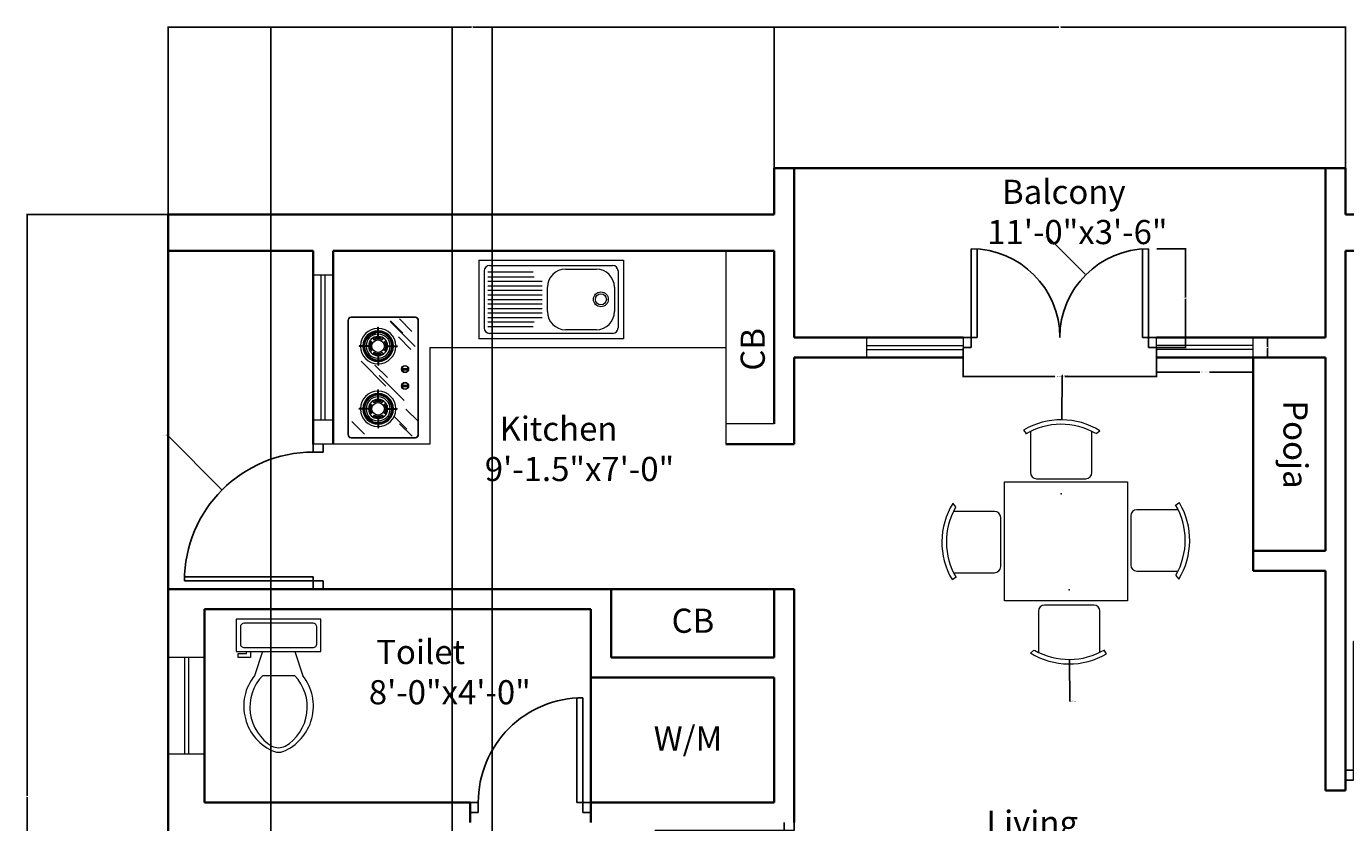
# Model space of a CAD drawing. Units: inches. Extents: x 3198 to 3702, y 1509 to 2253.
# Tile 5 of 6: x 3198 to 3526, y 2055 to 2253. Entities that reach past the tile are written whole.
import ezdxf

# ---------------------------------------------------------------- set-up
doc = ezdxf.new("R2010")
doc.units = ezdxf.units.IN
for name, color, linetype, lineweight in [('A-ANNO-DIMS', 2, 'Continuous', 18), ('A-ANNO-TEXT', 7, 'Continuous', 18), ('A-AREA-IDEN', 7, 'Continuous', 18), ('A-DOOR', 3, 'Continuous', 25), ('A-EQPM', 8, 'Continuous', 18), ('A-FLOR-CASE', 9, 'Continuous', 18), ('A-FLOR-FIXT', 9, 'Continuous', 18), ('A-FURN', 8, 'Continuous', 13), ('A-GLAZ', 4, 'Continuous', 18), ('A-WALL', 7, 'Continuous', 35)]:
    doc.layers.add(name, color=color, linetype=linetype, lineweight=lineweight)
doc.styles.get("Standard").update_dxf_attribs({"font": 'arial.ttf'})
doc.dimstyles.get("Standard").update_dxf_attribs({"dimtxt": 0.18, "dimasz": 0.18, "dimexe": 0.18, "dimexo": 0.0625, "dimgap": 0.09, "dimtad": 0, "dimtih": 1, "dimtoh": 1, "dimdec": 4, "dimzin": 0, "dimdsep": 46, "dimtxsty": 'Standard', "dimcen": 0.09, "dimadec": 0, "dimazin": 0, "dimtfac": 1, "dimtdec": 4, "dimtofl": 0, "dimtmove": 0, "dimatfit": 3, "dimfxl": 1, "dimtolj": 1, "dimtzin": 0, "dimarcsym": 0})

# ---------------------------------------------------------------- blocks, each defined once
blk = doc.blocks.new('A$C3E2236F0')
at = {"linetype": 'ByBlock'}
for p, q in [((0.639, 1.827), (0.658, 1.799)), ((0.692, 1.816), (0.692, 1.495)), ((1.172, 1.495), (1.172, 1.816)), ((1.207, 1.799), (1.235, 1.822)), ((0.74, 1.447), (1.124, 1.447)), ((0.489, 0.494), (0.489, 1.422)), ((0.489, 1.422), (1.452, 1.422)), ((1.452, 1.422), (1.452, 0.494)), ((0.108, 1.227), (0.085, 1.255)), ((1.857, 1.258), (1.829, 1.239)), ((0.412, 1.192), (0.091, 1.192)), ((0.46, 0.76), (0.46, 1.144)), ((1.477, 1.157), (1.477, 0.773)), ((1.846, 1.205), (1.525, 1.205)), ((1.525, 0.725), (1.846, 0.725)), ((0.08, 0.659), (0.108, 0.678)), ((0.091, 0.712), (0.412, 0.712)), ((1.829, 0.69), (1.852, 0.662)), ((1.452, 0.494), (0.489, 0.494)), ((1.187, 0.46), (0.803, 0.46)), ((0.755, 0.412), (0.755, 0.091)), ((1.235, 0.091), (1.235, 0.412)), ((0.72, 0.108), (0.692, 0.085)), ((1.288, 0.08), (1.269, 0.108))]:
    blk.add_line(p, q, dxfattribs=at)
for centre, radius, start, end in [((0.932, 1.328), 0.579, 58.5054, 120.4019), ((0.932, 1.328), 0.544, 60.0817, 120.6821), ((0.74, 1.495), 0.048, 180, 270), ((1.124, 1.495), 0.048, 270, 0), ((0.579, 0.952), 0.579, 148.5054, 210.4019), ((1.358, 0.965), 0.544, 330.0817, 30.6821), ((1.358, 0.965), 0.579, 328.5054, 30.4019), ((0.579, 0.952), 0.544, 150.0817, 210.6821), ((0.412, 1.144), 0.048, 0, 90), ((1.525, 1.157), 0.048, 90, 180), ((0.412, 0.76), 0.048, 270, 0), ((1.525, 0.773), 0.048, 180, 270), ((0.803, 0.412), 0.048, 90, 180), ((1.187, 0.412), 0.048, 0, 90), ((0.995, 0.579), 0.544, 240.0817, 300.6821), ((0.995, 0.579), 0.579, 238.5054, 300.4019)]:
    blk.add_arc(centre, radius, start, end, dxfattribs=at)
blk = doc.blocks.new('*U4')
for p, q in [((9.5, -6), (9.5, -2)), ((-10, -8.5), (-8, -8.5)), ((-10, -9.5), (-10, -8.5)), ((-7, -9.5), (-10, -9.5)), ((-8, -8.5), (-8, -8)), ((-7, -8), (-7, -9.5)), ((-4, -8), (-6, -14)), ((4, -8), (6, -14)), ((4, -14), (-4, -14))]:
    blk.add_line(p, q)
blk.add_lwpolyline([(10.5, -8), (10.5, 0), (-10.5, 0), (-10.5, -8)], close=True)
for points in [[(-9.5, -2), (-9.5, -6)], [(8.5, -1), (-8.5, -1)], [(-8.5, -7), (8.5, -7)]]:
    blk.add_lwpolyline(points)
for centre, radius, start, end in [((-8.62, -1.88), 0.884, 81.8699, 188.1301), ((8.62, -1.88), 0.884, 351.8699, 98.1301), ((-8.62, -6.12), 0.884, 171.8699, 278.1301), ((8.62, -6.12), 0.884, 261.8699, 8.1301), ((3.52, -21.58), 12.17, 141.4691, 247.9714), ((4.2, -21.82), 11.33, 136.3677, 238.9468), ((-3.52, -21.58), 12.17, 292.0284, 38.5307), ((-4.2, -21.82), 11.33, 301.053, 43.6321), ((0, -27.88), 4, 245.7318, 294.2682), ((0, -29), 4, 254.8605, 285.1395)]:
    blk.add_arc(centre, radius, start, end)
blk = doc.blocks.new('A$C48FA29D1')
for p, q in [((23.9, 336.8), (101.3, 414.2)), ((177.6, 369.5), (182.6, 369.5)), ((320.9, 202.7), (475.7, 357.5)), ((572.4, 369.5), (567.4, 369.5)), ((63.2, 254.2), (63.2, 249.2)), ((299, 254.2), (299, 249.2)), ((374.2, 193.8), (451.6, 271.2)), ((451, 254.2), (451, 249.2)), ((686.8, 254.2), (686.8, 249.2)), ((232.1, 89.3), (386.9, 244.1)), ((567.6, 22.2), (722.4, 177)), ((650.5, 97.2), (727.9, 174.6)), ((10.1, 41), (87.5, 118.4)), ((54.5, 73.5), (131.9, 150.9)), ((177.6, 133.3), (182.6, 133.3)), ((549.9, 47.9), (627.2, 125.3)), ((572.4, 133.3), (567.4, 133.3)), ((661.4, 42), (738.7, 119.3)), ((100.9, 1.5), (178.3, 78.9))]:
    blk.add_line(p, q)
at = {"ltscale": 0.18}
for p, q in [((177.6, 296.7), (177.6, 369.5)), ((182.6, 296.7), (182.6, 369.5)), ((567.4, 296.7), (567.4, 369.5)), ((572.4, 296.7), (572.4, 369.5)), ((135.1, 254.2), (63.2, 254.2)), ((135.1, 249.2), (63.2, 249.2)), ((126.9, 279.5), (132.1, 274.3)), ((131.2, 286.5), (142, 275.7)), ((145.3, 300.6), (156.1, 289.8)), ((152.3, 304.9), (157.6, 299.7)), ((202.6, 299.7), (207.8, 304.9)), ((204, 289.8), (214.8, 300.6)), ((218.2, 275.7), (229, 286.5)), ((225, 254.2), (299, 254.2)), ((225, 249.2), (299, 249.2)), ((228.1, 274.3), (233.3, 279.5)), ((525, 254.2), (451, 254.2)), ((525, 249.2), (451, 249.2)), ((521.9, 274.3), (516.7, 279.5)), ((531.8, 275.7), (521, 286.5)), ((546, 289.8), (535.2, 300.6)), ((547.4, 299.7), (542.2, 304.9)), ((597.7, 304.9), (592.4, 299.7)), ((604.7, 300.6), (593.9, 289.8)), ((618.8, 286.5), (608, 275.7)), ((614.9, 254.2), (686.8, 254.2)), ((614.9, 249.2), (686.8, 249.2)), ((623.1, 279.5), (617.9, 274.3)), ((126.9, 224), (132.1, 229.2)), ((131.2, 217), (142, 227.8)), ((145.3, 202.8), (156.1, 213.6)), ((152.3, 198.5), (157.6, 203.8)), ((177.6, 206.8), (177.6, 133.3)), ((182.6, 206.8), (182.6, 133.3)), ((202.6, 203.8), (207.8, 198.5)), ((204, 213.6), (214.8, 202.8)), ((218.2, 227.8), (229, 217)), ((228.1, 229.2), (233.3, 224)), ((521.9, 229.2), (516.7, 224)), ((531.8, 227.8), (521, 217)), ((546, 213.6), (535.2, 202.8)), ((547.4, 203.8), (542.2, 198.5)), ((567.4, 206.8), (567.4, 133.3)), ((572.4, 206.8), (572.4, 133.3)), ((597.7, 198.5), (592.4, 203.8)), ((604.7, 202.8), (593.9, 213.6)), ((618.8, 217), (608, 227.8)), ((623.1, 224), (617.9, 229.2)), ((318.6, 99.8), (318.6, 69)), ((326.6, 99.8), (326.6, 69)), ((423.4, 99.8), (423.4, 69)), ((431.4, 99.8), (431.4, 69))]:
    blk.add_line(p, q, dxfattribs=at)
for points in [[(20, 0), (730, 0, 0.414214), (750, 20), (750, 420, 0.414214), (730, 440), (20, 440, 0.414214), (0, 420), (0, 20, 0.414214)], [(20, 3), (730, 3, 0.414214), (747, 20), (747, 420, 0.414214), (730, 437), (20, 437, 0.414214), (3, 420), (3, 20, 0.414214)]]:
    blk.add_lwpolyline(points, format="xyb", close=True)
for centre in [(109.4, 291.3), (115.3, 300.3), (642.8, 283.6), (646.9, 273)]:
    blk.add_circle(centre, 3.58)
for centre, radius in [((180.1, 251.7), 39), ((569.9, 251.7), 39), ((322.6, 84.4), 22.5), ((322.6, 84.4), 21.5), ((427.4, 84.4), 22.5), ((427.4, 84.4), 21.5)]:
    blk.add_circle(centre, radius, dxfattribs=at)
for centre, radius, start, end in [((180.1, 251.7), 110, 91.30229, 178.69771), ((180.1, 251.7), 95, 91.59175, 178.40825), ((180.1, 251.7), 90, 91.59175, 178.40825), ((180.1, 251.7), 85, 91.68541, 178.31459), ((180.1, 251.7), 110, 1.30229, 88.69771), ((180.1, 251.7), 90, 1.59175, 88.40825), ((180.1, 251.7), 85, 1.68541, 88.31459), ((180.1, 251.7), 95, 1.59175, 88.40825), ((569.9, 251.7), 110, 91.30229, 178.69771), ((569.9, 251.7), 95, 91.59175, 178.40825), ((569.9, 251.7), 90, 91.59175, 178.40825), ((569.9, 251.7), 85, 91.68541, 178.31459), ((569.9, 251.7), 110, 1.30229, 88.69771), ((569.9, 251.7), 90, 1.59175, 88.40825), ((569.9, 251.7), 85, 1.68541, 88.31459), ((569.9, 251.7), 95, 1.59175, 88.40825), ((180.1, 251.7), 110, 181.30229, 268.69771), ((180.1, 251.7), 95, 181.59175, 268.40825), ((180.1, 251.7), 90, 181.59175, 268.40825), ((180.1, 251.7), 85, 181.68541, 268.31459), ((180.1, 251.7), 75, 91.91021, 178.08979), ((180.1, 251.7), 75, 181.91021, 268.08979), ((180.1, 251.7), 60, 92.38802, 177.61198), ((180.1, 251.7), 60, 182.38802, 267.61198), ((180.1, 251.7), 53, 154.85389, 177.29637), ((180.1, 251.7), 53, 182.70363, 205.14611), ((180.1, 251.7), 45, 147.83959, 176.81526), ((134.3, 251.7), 2.64, 288.75105, 71.24895), ((180.1, 251.7), 45, 183.18474, 212.16041), ((180.1, 251.7), 45, 93.18474, 122.16041), ((180.1, 251.7), 53, 92.70363, 115.14611), ((180.1, 297), 2.52, 186.73537, 353.26463), ((180.1, 251.7), 75, 1.91021, 88.08979), ((180.1, 251.7), 60, 2.38802, 87.61198), ((180.1, 251.7), 53, 64.85389, 87.29637), ((180.1, 251.7), 45, 57.83959, 86.81526), ((180.1, 251.7), 90, 271.59175, 358.40825), ((180.1, 251.7), 85, 271.68541, 358.31459), ((180.1, 251.7), 110, 271.30229, 358.69771), ((180.1, 251.7), 75, 271.91021, 358.08979), ((180.1, 251.7), 60, 272.38802, 357.61198), ((180.1, 251.7), 95, 271.59175, 358.40825), ((180.1, 251.7), 45, 3.18474, 32.16041), ((180.1, 251.7), 45, 327.83959, 356.81526), ((225.9, 251.7), 2.67, 110.55069, 249.44931), ((180.1, 251.7), 53, 2.70363, 25.14611), ((180.1, 251.7), 53, 334.85389, 357.29637), ((569.9, 251.7), 110, 181.30229, 268.69771), ((569.9, 251.7), 95, 181.59175, 268.40825), ((569.9, 251.7), 90, 181.59175, 268.40825), ((569.9, 251.7), 85, 181.68541, 268.31459), ((569.9, 251.7), 75, 91.91021, 178.08979), ((569.9, 251.7), 75, 181.91021, 268.08979), ((569.9, 251.7), 60, 92.38802, 177.61198), ((569.9, 251.7), 60, 182.38802, 267.61198), ((569.9, 251.7), 53, 154.85389, 177.29637), ((569.9, 251.7), 53, 182.70363, 205.14611), ((569.9, 251.7), 45, 147.83959, 176.81526), ((524.2, 251.7), 2.63, 288.41197, 71.58803), ((569.9, 251.7), 45, 183.18474, 212.16041), ((569.9, 251.7), 45, 93.18474, 122.16041), ((569.9, 251.7), 53, 92.70363, 115.14611), ((569.9, 296.8), 2.51, 183.95793, 356.04207), ((569.9, 251.7), 75, 1.91021, 88.08979), ((569.9, 251.7), 60, 2.38802, 87.61198), ((569.9, 251.7), 53, 64.85389, 87.29637), ((569.9, 251.7), 45, 57.83959, 86.81526), ((569.9, 251.7), 75, 271.91021, 358.08979), ((569.9, 251.7), 85, 271.68541, 358.31459), ((569.9, 251.7), 110, 271.30229, 358.69771), ((569.9, 251.7), 90, 271.59175, 358.40825), ((569.9, 251.7), 60, 272.38802, 357.61198), ((569.9, 251.7), 95, 271.59175, 358.40825), ((569.9, 251.7), 45, 3.18474, 32.16041), ((569.9, 251.7), 45, 327.83959, 356.81526), ((615.5, 251.7), 2.58, 104.29448, 255.70552), ((569.9, 251.7), 53, 2.70363, 25.14611), ((569.9, 251.7), 53, 334.85389, 357.29637), ((180.1, 251.7), 45, 237.83959, 266.81526), ((180.1, 251.7), 53, 244.85389, 267.29637), ((180.1, 205.8), 2.69, 21.78852, 158.21148), ((180.1, 251.7), 45, 273.18474, 302.16041), ((180.1, 251.7), 53, 272.70363, 295.14611), ((569.9, 251.7), 45, 237.83959, 266.81526), ((569.9, 251.7), 53, 244.85389, 267.29637), ((569.9, 206), 2.63, 17.9418, 162.0582), ((569.9, 251.7), 45, 273.18474, 302.16041), ((569.9, 251.7), 53, 272.70363, 295.14611), ((322.6, 84.4), 18.5, 111.32369, 248.67631), ((316.6, 99.8), 2, 0, 111.32369), ((328.6, 99.8), 2, 68.67631, 180), ((322.6, 84.4), 18.5, 291.32369, 68.67631), ((427.4, 84.4), 18.5, 111.32369, 248.67631), ((421.4, 99.8), 2, 0, 111.32369), ((433.4, 99.8), 2, 68.67631, 180), ((427.4, 84.4), 18.5, 291.32369, 68.67631), ((316.6, 69), 2, 248.67631, 0), ((328.6, 69), 2, 180, 291.32369), ((421.4, 69), 2, 248.67631, 0), ((433.4, 69), 2, 180, 291.32369)]:
    blk.add_arc(centre, radius, start, end, dxfattribs=at)
blk = doc.blocks.new('A$C56104318')
for p, q in [((0, 0.609), (1.12, 0.609)), ((0, 0.609), (0, 0)), ((0.042, 0.525), (0.042, 0.084)), ((0.42, 0.515), (0.07, 0.515)), ((0.084, 0.567), (1.036, 0.567)), ((0.672, 0.539), (0.91, 0.539)), ((1.078, 0.525), (1.078, 0.084)), ((1.12, 0.609), (1.12, 0)), ((0.07, 0.48), (0.429, 0.48)), ((0.07, 0.445), (0.49, 0.445)), ((0.07, 0.41), (0.49, 0.41)), ((0.07, 0.375), (0.49, 0.375)), ((0.07, 0.34), (0.49, 0.34)), ((0.532, 0.21), (0.532, 0.399)), ((1.05, 0.399), (1.05, 0.21)), ((0.07, 0.305), (0.49, 0.305)), ((0.07, 0.27), (0.49, 0.27)), ((0.07, 0.235), (0.49, 0.235)), ((0.07, 0.2), (0.49, 0.2)), ((0.07, 0.165), (0.49, 0.165)), ((0.07, 0.13), (0.429, 0.13)), ((0.07, 0.094), (0.42, 0.094)), ((1.036, 0.042), (0.084, 0.042)), ((0.91, 0.07), (0.672, 0.07)), ((1.12, 0), (0, 0))]:
    blk.add_line(p, q)
for radius in [0.0574, 0.0427]:
    blk.add_circle((0.945, 0.305), radius)
for centre, radius, start, end in [((0.084, 0.525), 0.042, 90, 180), ((0.672, 0.399), 0.14, 90, 180), ((0.91, 0.399), 0.14, 0, 90), ((1.036, 0.525), 0.042, 0, 90), ((0.672, 0.21), 0.14, 180, 270), ((0.91, 0.21), 0.14, 270, 0), ((0.084, 0.084), 0.042, 180, 270), ((1.036, 0.084), 0.042, 270, 0)]:
    blk.add_arc(centre, radius, start, end)
blk = doc.blocks.new('A$C559B0E78')
at = {"xscale": 729, "yscale": 729, "zscale": 729}
blk.add_blockref('A$C56104318', (0, 0), dxfattribs=at)
blk = doc.blocks.new('DOOR-SINGLE-32')
for p, q in [((0, 34), (32, 34)), ((32, 36), (32, 34)), ((32, 34), (34.5, 34)), ((32, 32.5), (32, 34)), ((34.5, 34), (34.5, 36)), ((0.04, 32.5), (32, 32.5)), ((32, 0), (32, 2)), ((32, 2), (34.5, 2)), ((34.5, 2), (34.5, 0))]:
    blk.add_line(p, q)
blk.add_arc((32, 34), 32, 180, 270)
blk = doc.blocks.new('DOOR-SINGLE-26')
for p, q in [((0, 30), (0, 28)), ((2.5, 28), (2.5, 30)), ((0, 28), (2.5, 28)), ((2.5, 28), (28.5, 28)), ((2.5, 28), (2.5, 26.5)), ((2.5, 26.5), (28.46, 26.5)), ((0, 0), (0, 2)), ((0, 2), (2.5, 2)), ((2.5, 2), (2.5, 0))]:
    blk.add_line(p, q)
blk.add_arc((2.5, 28), 26, 270, 0)
blk = doc.blocks.new('DOOR-BALCONY-PAIR-44')
for p, q in [((2, 2.5), (2, 24.5)), ((3.5, 2.5), (3.5, 24.45)), ((44.5, 2.5), (44.5, 24.45)), ((46, 2.5), (46, 24.5)), ((2, 2.5), (0, 2.5)), ((0, 0), (2, 0)), ((2, 0), (2, 2.5)), ((2, 2.5), (3.5, 2.5)), ((44.5, 2.5), (46, 2.5)), ((46, 0), (46, 2.5)), ((46, 2.5), (48, 2.5)), ((48, 0), (46, 0))]:
    blk.add_line(p, q)
for centre, start, end in [((2, 2.5), 0, 90), ((46, 2.5), 90, 180)]:
    blk.add_arc(centre, 22, start, end)
blk = doc.blocks.new('WIN-24-W9')
for p, q in [((9, 24), (0, 24)), ((4, 24), (4, 0)), ((5, 24), (5, 0)), ((9, 0), (0, 0))]:
    blk.add_line(p, q)
blk = doc.blocks.new('WIN-SIDELIGHT-24')
for p, q in [((0, 5), (0, 0)), ((24, 5), (24, 0)), ((0, 3), (24, 3)), ((0, 2), (24, 2))]:
    blk.add_line(p, q)
blk = doc.blocks.new('WIN-36-W5')
for p, q in [((0, 36), (5, 36)), ((2, 0), (2, 36)), ((3, 0), (3, 36)), ((0, 0), (5, 0))]:
    blk.add_line(p, q)
blk = doc.blocks.new('*D27')
at = {"layer": 'A-ANNO-DIMS', "color": 0, "lineweight": -2, "transparency": 16777216}
for p, q in [((3478.55, 2170.33), (3478.55, 2166.61)), ((3502.55, 2170.33), (3502.55, 2166.61)), ((3478.73, 2166.79), (3489.32, 2166.79)), ((3502.37, 2166.79), (3491.77, 2166.79))]:
    blk.add_line(p, q, dxfattribs=at)
at = {"layer": 'A-ANNO-DIMS', "color": 0, "transparency": 16777216}
for points in [[(3478.73, 2166.82), (3478.73, 2166.76), (3478.55, 2166.79)], [(3502.37, 2166.82), (3502.37, 2166.76), (3502.55, 2166.79)]]:
    blk.add_solid(points, dxfattribs=at)
at = {"layer": 'Defpoints', "color": 0, "transparency": 16777216}
for p in [(3478.55, 2170.39), (3502.55, 2170.39), (3478.55, 2166.79)]:
    blk.add_point(p, dxfattribs=at)
at = {"layer": 'A-ANNO-DIMS', "color": 0, "transparency": 16777216, "insert": (3490.55, 2166.79), "char_height": 0.18, "attachment_point": 5}
blk.add_mtext('\\A1;SIDELIGHT 24 TYP.', dxfattribs=at)
blk = doc.blocks.new('*D28')
at = {"layer": 'A-ANNO-DIMS', "color": 0, "lineweight": -2, "transparency": 16777216}
for p, q in [((3502.61, 2175.39), (3506.33, 2175.39)), ((3506.15, 2175.21), (3506.15, 2173.07)), ((3502.61, 2170.39), (3506.33, 2170.39)), ((3506.15, 2170.57), (3506.15, 2172.71))]:
    blk.add_line(p, q, dxfattribs=at)
at = {"layer": 'A-ANNO-DIMS', "color": 0, "transparency": 16777216}
for points in [[(3506.12, 2175.21), (3506.18, 2175.21), (3506.15, 2175.39)], [(3506.12, 2170.57), (3506.18, 2170.57), (3506.15, 2170.39)]]:
    blk.add_solid(points, dxfattribs=at)
at = {"layer": 'Defpoints', "color": 0, "transparency": 16777216}
for p in [(3502.55, 2175.39), (3502.55, 2170.39), (3506.15, 2170.39)]:
    blk.add_point(p, dxfattribs=at)
at = {"layer": 'A-ANNO-DIMS', "color": 0, "transparency": 16777216, "insert": (3506.15, 2172.89), "char_height": 0.18, "attachment_point": 5}
blk.add_mtext('\\A1;5 TYP.', dxfattribs=at)
blk = doc.blocks.new('*D37')
at = {"layer": 'A-ANNO-DIMS', "color": 0, "lineweight": -2, "transparency": 16777216}
for p, q in [((3430.55, 2172.83), (3430.55, 2165.51)), ((3478.55, 2172.83), (3478.55, 2165.51)), ((3430.73, 2165.69), (3453.28, 2165.69)), ((3478.37, 2165.69), (3455.81, 2165.69))]:
    blk.add_line(p, q, dxfattribs=at)
at = {"layer": 'A-ANNO-DIMS', "color": 0, "transparency": 16777216}
for points in [[(3430.73, 2165.72), (3430.73, 2165.66), (3430.55, 2165.69)], [(3478.37, 2165.72), (3478.37, 2165.66), (3478.55, 2165.69)]]:
    blk.add_solid(points, dxfattribs=at)
at = {"layer": 'Defpoints', "color": 0, "transparency": 16777216}
for p in [(3430.55, 2172.89), (3478.55, 2172.89), (3478.55, 2165.69)]:
    blk.add_point(p, dxfattribs=at)
at = {"layer": 'A-ANNO-DIMS', "color": 0, "transparency": 16777216, "insert": (3454.55, 2165.69), "char_height": 0.18, "attachment_point": 5}
blk.add_mtext('\\A1;DOOR PAIR 48 TYP.', dxfattribs=at)
blk = doc.blocks.new('*D38')
at = {"layer": 'A-ANNO-DIMS', "color": 0, "lineweight": -2, "transparency": 16777216}
for p, q in [((3478.61, 2197.39), (3485.93, 2197.39)), ((3485.75, 2197.21), (3485.75, 2185.32)), ((3485.75, 2173.07), (3485.75, 2184.96)), ((3478.61, 2172.89), (3485.93, 2172.89))]:
    blk.add_line(p, q, dxfattribs=at)
at = {"layer": 'A-ANNO-DIMS', "color": 0, "transparency": 16777216}
for points in [[(3485.72, 2197.21), (3485.78, 2197.21), (3485.75, 2197.39)], [(3485.72, 2173.07), (3485.78, 2173.07), (3485.75, 2172.89)]]:
    blk.add_solid(points, dxfattribs=at)
at = {"layer": 'Defpoints', "color": 0, "transparency": 16777216}
for p in [(3478.55, 2197.39), (3485.75, 2197.39), (3478.55, 2172.89)]:
    blk.add_point(p, dxfattribs=at)
at = {"layer": 'A-ANNO-DIMS', "color": 0, "transparency": 16777216, "insert": (3485.75, 2185.14), "char_height": 0.18, "attachment_point": 5}
blk.add_mtext('\\A1;25 TYP.', dxfattribs=at)
blk = doc.blocks.new('*D45')
at = {"layer": 'A-ANNO-DIMS', "color": 0, "lineweight": -2, "transparency": 16777216}
for p, q in [((3233.05, 2205.95), (3233.05, 2252.62)), ((3233.23, 2252.44), (3307.91, 2252.44)), ((3383.37, 2252.44), (3308.68, 2252.44)), ((3383.55, 2205.95), (3383.55, 2252.62))]:
    blk.add_line(p, q, dxfattribs=at)
at = {"layer": 'A-ANNO-DIMS', "color": 0, "transparency": 16777216}
for points in [[(3233.23, 2252.47), (3233.23, 2252.41), (3233.05, 2252.44)], [(3383.37, 2252.47), (3383.37, 2252.41), (3383.55, 2252.44)]]:
    blk.add_solid(points, dxfattribs=at)
at = {"layer": 'Defpoints', "color": 0, "transparency": 16777216}
for p in [(3383.55, 2252.44), (3233.05, 2205.89), (3383.55, 2205.89)]:
    blk.add_point(p, dxfattribs=at)
at = {"layer": 'A-ANNO-DIMS', "color": 0, "transparency": 16777216, "insert": (3308.3, 2252.44), "char_height": 0.18, "attachment_point": 5}
blk.add_mtext('\\A1;150.5', dxfattribs=at)
blk = doc.blocks.new('*D46')
at = {"layer": 'A-ANNO-DIMS', "color": 0, "lineweight": -2, "transparency": 16777216}
for p, q in [((3383.55, 2217.45), (3383.55, 2252.62)), ((3383.73, 2252.44), (3454.27, 2252.44)), ((3525.37, 2252.44), (3454.83, 2252.44)), ((3525.55, 2217.45), (3525.55, 2252.62))]:
    blk.add_line(p, q, dxfattribs=at)
at = {"layer": 'A-ANNO-DIMS', "color": 0, "transparency": 16777216}
for points in [[(3383.73, 2252.47), (3383.73, 2252.41), (3383.55, 2252.44)], [(3525.37, 2252.47), (3525.37, 2252.41), (3525.55, 2252.44)]]:
    blk.add_solid(points, dxfattribs=at)
at = {"layer": 'Defpoints', "color": 0, "transparency": 16777216}
for p in [(3525.55, 2252.44), (3383.55, 2217.39), (3525.55, 2217.39)]:
    blk.add_point(p, dxfattribs=at)
at = {"layer": 'A-ANNO-DIMS', "color": 0, "transparency": 16777216, "insert": (3454.55, 2252.44), "char_height": 0.18, "attachment_point": 5}
blk.add_mtext('\\A1;142', dxfattribs=at)
blk = doc.blocks.new('*D48')
at = {"layer": 'A-ANNO-DIMS', "color": 0, "lineweight": -2, "transparency": 16777216}
for p, q in [((3232.98, 2205.89), (3197.82, 2205.89)), ((3198, 2205.71), (3198, 2061.57)), ((3198, 1917.07), (3198, 2061.21)), ((3232.98, 1916.89), (3197.82, 1916.89))]:
    blk.add_line(p, q, dxfattribs=at)
at = {"layer": 'A-ANNO-DIMS', "color": 0, "transparency": 16777216}
for points in [[(3197.97, 2205.71), (3198.03, 2205.71), (3198, 2205.89)], [(3197.97, 1917.07), (3198.03, 1917.07), (3198, 1916.89)]]:
    blk.add_solid(points, dxfattribs=at)
at = {"layer": 'Defpoints', "color": 0, "transparency": 16777216}
for p in [(3233.05, 2205.89), (3198, 1916.89), (3233.05, 1916.89)]:
    blk.add_point(p, dxfattribs=at)
at = {"layer": 'A-ANNO-DIMS', "color": 0, "transparency": 16777216, "insert": (3198, 2061.39), "char_height": 0.18, "attachment_point": 5}
blk.add_mtext('\\A1;289', dxfattribs=at)
blk = doc.blocks.new('*D53')
at = {"layer": 'A-ANNO-DIMS', "color": 0, "lineweight": -2, "transparency": 16777216}
for p, q in [((3233.05, 1916.95), (3233.05, 2252.62)), ((3233.23, 2252.44), (3245.47, 2252.44)), ((3258.37, 2252.44), (3246.12, 2252.44)), ((3258.55, 1916.95), (3258.55, 2252.62))]:
    blk.add_line(p, q, dxfattribs=at)
at = {"layer": 'A-ANNO-DIMS', "color": 0, "transparency": 16777216}
for points in [[(3233.23, 2252.47), (3233.23, 2252.41), (3233.05, 2252.44)], [(3258.37, 2252.47), (3258.37, 2252.41), (3258.55, 2252.44)]]:
    blk.add_solid(points, dxfattribs=at)
at = {"layer": 'Defpoints', "color": 0, "transparency": 16777216}
for p in [(3258.55, 2252.44), (3233.05, 1916.89), (3258.55, 1916.89)]:
    blk.add_point(p, dxfattribs=at)
at = {"layer": 'A-ANNO-DIMS', "color": 0, "transparency": 16777216, "insert": (3245.8, 2252.44), "char_height": 0.18, "attachment_point": 5}
blk.add_mtext('\\A1;25.5', dxfattribs=at)
blk = doc.blocks.new('*D54')
at = {"layer": 'A-ANNO-DIMS', "color": 0, "lineweight": -2, "transparency": 16777216}
for p, q in [((3303.55, 1916.95), (3303.55, 2252.62)), ((3303.73, 2252.44), (3308.34, 2252.44)), ((3313.37, 2252.44), (3308.76, 2252.44)), ((3313.55, 1916.95), (3313.55, 2252.62))]:
    blk.add_line(p, q, dxfattribs=at)
at = {"layer": 'A-ANNO-DIMS', "color": 0, "transparency": 16777216}
for points in [[(3303.73, 2252.47), (3303.73, 2252.41), (3303.55, 2252.44)], [(3313.37, 2252.47), (3313.37, 2252.41), (3313.55, 2252.44)]]:
    blk.add_solid(points, dxfattribs=at)
at = {"layer": 'Defpoints', "color": 0, "transparency": 16777216}
for p in [(3313.55, 2252.44), (3303.55, 1916.89), (3313.55, 1916.89)]:
    blk.add_point(p, dxfattribs=at)
at = {"layer": 'A-ANNO-DIMS', "color": 0, "transparency": 16777216, "insert": (3308.55, 2252.44), "char_height": 0.18, "attachment_point": 5}
blk.add_mtext('\\A1;10', dxfattribs=at)
blk = doc.blocks.new('*D61')
at = {"layer": 'A-ANNO-DIMS', "color": 0, "lineweight": -2, "transparency": 16777216}
for p, q in [((3232.66, 2151.09), (3232.84, 2151.09)), ((3232.84, 2151.09), (3246.29, 2137.64)), ((3268.96, 2114.89), (3269.14, 2114.89)), ((3269.05, 2114.8), (3269.05, 2114.98))]:
    blk.add_line(p, q, dxfattribs=at)
at = {"layer": 'A-ANNO-DIMS', "color": 0, "transparency": 16777216}
blk.add_solid([(3246.31, 2137.66), (3246.27, 2137.62), (3246.42, 2137.52)], dxfattribs=at)
at = {"layer": 'Defpoints', "color": 0, "transparency": 16777216}
for p in [(3246.42, 2137.52), (3269.05, 2114.89)]:
    blk.add_point(p, dxfattribs=at)
at = {"layer": 'A-ANNO-DIMS', "color": 0, "transparency": 16777216, "insert": (3232.17, 2151.09), "char_height": 0.18, "attachment_point": 5}
blk.add_mtext('\\A1;9X R32', dxfattribs=at)
blk = doc.blocks.new('*D63')
at = {"layer": 'A-ANNO-DIMS', "color": 0, "lineweight": -2, "transparency": 16777216}
for p, q in [((3451.48, 2200.28), (3451.66, 2200.28)), ((3451.66, 2200.28), (3460.86, 2191.07)), ((3476.46, 2175.39), (3476.64, 2175.39)), ((3476.55, 2175.3), (3476.55, 2175.48))]:
    blk.add_line(p, q, dxfattribs=at)
at = {"layer": 'A-ANNO-DIMS', "color": 0, "transparency": 16777216}
blk.add_solid([(3460.88, 2191.09), (3460.84, 2191.05), (3460.99, 2190.94)], dxfattribs=at)
at = {"layer": 'Defpoints', "color": 0, "transparency": 16777216}
for p in [(3460.99, 2190.94), (3476.55, 2175.39)]:
    blk.add_point(p, dxfattribs=at)
at = {"layer": 'A-ANNO-DIMS', "color": 0, "transparency": 16777216, "insert": (3450.98, 2200.28), "char_height": 0.18, "attachment_point": 5}
blk.add_mtext('\\A1;4X R22', dxfattribs=at)
blk = doc.blocks.new('*D64')
at = {"layer": 'A-ANNO-DIMS', "color": 0, "lineweight": -2, "transparency": 16777216}
for p, q in [((3455.15, 2165.95), (3455.05, 2155.09)), ((3455.33, 2165.95), (3455.15, 2165.95)), ((3454.78, 2136.51), (3454.96, 2136.51)), ((3454.87, 2136.42), (3454.87, 2136.6))]:
    blk.add_line(p, q, dxfattribs=at)
at = {"layer": 'A-ANNO-DIMS', "color": 0, "transparency": 16777216}
blk.add_solid([(3455.02, 2155.09), (3455.08, 2155.09), (3455.05, 2154.91)], dxfattribs=at)
at = {"layer": 'Defpoints', "color": 0, "transparency": 16777216}
for p in [(3455.05, 2154.91), (3454.87, 2136.51)]:
    blk.add_point(p, dxfattribs=at)
at = {"layer": 'A-ANNO-DIMS', "color": 0, "transparency": 16777216, "insert": (3455.93, 2165.95), "char_height": 0.18, "attachment_point": 5}
blk.add_mtext('\\A1;8X R18.4', dxfattribs=at)
blk = doc.blocks.new('*D65')
at = {"layer": 'A-ANNO-DIMS', "color": 0, "lineweight": -2, "transparency": 16777216}
for p, q in [((3456.77, 2112.7), (3456.95, 2112.7)), ((3456.86, 2112.61), (3456.86, 2112.79)), ((3457.04, 2085.04), (3456.98, 2095.23)), ((3457.22, 2085.04), (3457.04, 2085.04))]:
    blk.add_line(p, q, dxfattribs=at)
at = {"layer": 'A-ANNO-DIMS', "color": 0, "transparency": 16777216}
blk.add_solid([(3457.01, 2095.23), (3456.95, 2095.23), (3456.98, 2095.41)], dxfattribs=at)
at = {"layer": 'Defpoints', "color": 0, "transparency": 16777216}
for p in [(3456.86, 2112.7), (3456.98, 2095.41)]:
    blk.add_point(p, dxfattribs=at)
at = {"layer": 'A-ANNO-DIMS', "color": 0, "transparency": 16777216, "insert": (3457.97, 2085.04), "char_height": 0.18, "attachment_point": 5}
blk.add_mtext('\\A1;8X R17.286', dxfattribs=at)

msp = doc.modelspace()

# ---------------------------------------------------------------- linework, layer by layer
at = {"layer": 'A-DOOR'}
for p, q in [((3269.0475, 2148.888), (3269.0475, 2146.888)), ((3269.0475, 2146.888), (3271.5475, 2146.888)), ((3271.5475, 2146.888), (3271.5475, 2148.888)), ((3269.0475, 2114.888), (3237.0475, 2114.888)), ((3269.0475, 2115.888), (3237.0631, 2115.888)), ((3269.0475, 2114.888), (3269.0475, 2115.888)), ((3269.0475, 2112.888), (3269.0475, 2114.888)), ((3269.0475, 2114.888), (3271.5475, 2114.888)), ((3271.5475, 2114.888), (3271.5475, 2112.888))]:
    msp.add_line(p, q, dxfattribs=at)
msp.add_arc((3269.0475, 2114.888), 32, 90, 180, dxfattribs=at)
at = {"layer": 'A-FLOR-CASE'}
for p, q in [((3371.5475, 2196.888), (3371.5475, 2148.888)), ((3298.0475, 2172.888), (3371.5475, 2172.888)), ((3298.0475, 2172.888), (3298.0475, 2148.888)), ((3383.5475, 2153.888), (3371.5475, 2153.888)), ((3298.0475, 2148.888), (3269.0475, 2148.888))]:
    msp.add_line(p, q, dxfattribs=at)
at = {"layer": 'A-WALL'}
for p, q in [((3383.5475, 2217.388), (3383.5475, 2205.888)), ((3383.5475, 2217.388), (3525.5475, 2217.388)), ((3388.5475, 2217.388), (3388.5475, 2175.388)), ((3520.5475, 2217.388), (3520.5475, 2175.388)), ((3525.5475, 2217.388), (3525.5475, 2205.888)), ((3233.0475, 2205.888), (3233.0475, 1916.888)), ((3233.0475, 2205.888), (3383.5475, 2205.888)), ((3525.5475, 2205.888), (3666.5475, 2205.888)), ((3233.0475, 2196.888), (3269.0475, 2196.888)), ((3269.0475, 2196.888), (3269.0475, 2148.888)), ((3274.0475, 2196.888), (3274.0475, 2148.888)), ((3274.0475, 2196.888), (3383.5475, 2196.888)), ((3383.5475, 2196.888), (3383.5475, 2153.888)), ((3525.5475, 2196.888), (3657.5475, 2196.888)), ((3525.5475, 2196.888), (3525.5475, 2062.888)), ((3388.5475, 2175.388), (3430.5475, 2175.388)), ((3478.5475, 2175.388), (3520.5475, 2175.388)), ((3388.5475, 2170.388), (3430.5475, 2170.388)), ((3388.5475, 2170.388), (3388.5475, 2148.888)), ((3478.5475, 2170.388), (3520.5475, 2170.388)), ((3502.5475, 2170.388), (3502.5475, 2117.388)), ((3520.5475, 2170.388), (3520.5475, 2122.388)), ((3388.5475, 2148.888), (3371.5475, 2148.888)), ((3502.5475, 2122.388), (3520.5475, 2122.388)), ((3502.5475, 2117.388), (3520.5475, 2117.388)), ((3520.5475, 2117.388), (3520.5475, 2062.888)), ((3388.5475, 2112.888), (3233.0475, 2112.888)), ((3343.0475, 2112.888), (3343.0475, 2095.888)), ((3383.5475, 2112.888), (3383.5475, 2095.888)), ((3388.5475, 2112.888), (3388.5475, 2054.888)), ((3242.0475, 2107.888), (3338.0475, 2107.888)), ((3242.0475, 2107.888), (3242.0475, 2059.888)), ((3338.0475, 2107.888), (3338.0475, 2054.888)), ((3343.0475, 2095.888), (3383.5475, 2095.888)), ((3338.0475, 2090.888), (3383.5475, 2090.888)), ((3383.5475, 2090.888), (3383.5475, 2059.888)), ((3520.5475, 2062.888), (3525.5475, 2062.888)), ((3242.0475, 2059.888), (3308.0475, 2059.888)), ((3308.0475, 2059.888), (3308.0475, 2054.888)), ((3338.0475, 2059.888), (3383.5475, 2059.888))]:
    msp.add_line(p, q, dxfattribs=at)

# ---------------------------------------------------------------- block references
at = {"layer": 'A-DOOR'}
for name, p in [('DOOR-BALCONY-PAIR-44', (3430.547, 2172.888)), ('DOOR-SINGLE-32', (3354.047, 2018.888))]:
    msp.add_blockref(name, p, dxfattribs=at)
at = {"layer": 'A-DOOR', "extrusion": (0, 0, -1), "zscale": -1}
for name, p, rotation in [('DOOR-SINGLE-32', (-3561.5475, 2099.8885), 269.9999999999991), ('DOOR-SINGLE-26', (-3308.0475, 2057.3875), 89.99999999999683)]:
    msp.add_blockref(name, p, dxfattribs=dict(at, rotation=rotation))
at = {"layer": 'A-EQPM', "xscale": 0.0399671811988082, "yscale": 0.0399671811988082, "zscale": 0.0399671811988082, "rotation": 90}
msp.add_blockref('A$C48FA29D1', (3295.2355, 2150.4366), dxfattribs=at)
at = {"layer": 'A-FLOR-FIXT', "xscale": 0.0440205214597798, "yscale": 0.0440205214597798, "zscale": 0.0440205214597798}
msp.add_blockref('A$C559B0E78', (3310.1909, 2175.0409), dxfattribs=at)
at = {"layer": 'A-FLOR-FIXT'}
msp.add_blockref('*U4', (3260.4496, 2105.3767), dxfattribs=at)
at = {"layer": 'A-FURN', "xscale": 31.78702146954402, "yscale": 31.78702146954402, "zscale": 31.78702146954402}
msp.add_blockref('A$C3E2236F0', (3425.239, 2094.2974), dxfattribs=at)
at = {"layer": 'A-GLAZ'}
for name, p in [('WIN-36-W5', (3269.047, 2154.888)), ('WIN-SIDELIGHT-24', (3406.547, 2170.388)), ('WIN-24-W9', (3233.047, 2071.888))]:
    msp.add_blockref(name, p, dxfattribs=at)
at = {"layer": 'A-GLAZ', "rotation": 180}
msp.add_blockref('WIN-SIDELIGHT-24', (3502.5479, 2175.388), dxfattribs=at)

# ---------------------------------------------------------------- texts
at = {"layer": 'A-ANNO-TEXT', "insert": (3375.2499, 2167.1123), "char_height": 6, "attachment_point": 1, "rotation": 90}
msp.add_mtext_dynamic_manual_height_columns('CB', width=32.112851, gutter_width=12.5, heights=[0], dxfattribs=at)
at = {"layer": 'A-ANNO-TEXT', "char_height": 6, "attachment_point": 1}
for s, insert in [('CB', (3358.0943, 2108.0238)), ('W/M', (3353.6464, 2078.7923))]:
    msp.add_mtext_dynamic_manual_height_columns(s, width=32.112851, gutter_width=12.5, heights=[0], dxfattribs=dict(at, insert=insert))
at = {"layer": 'A-AREA-IDEN', "attachment_point": 1}
for s, width, insert, char_height in [('  Balcony\\P11\'-0"x3\'-6"', 59.912118, (3436.5154, 2214.5443), 6), ('  Kitchen\\P9\'-1.5"x7\'-0"', 37.305441, (3311.6808, 2155.7078), 6), (' Toilet\\P8\'-0"x4\'-0"', 32.112851, (3282.8686, 2100.2644), 6), ('{\\H2.4x;      Living\\P11\'-0"x20\'-4.5"}', 72.249028, (3425.2579, 2057.8436), 2.5)]:
    msp.add_mtext_dynamic_manual_height_columns(s, width=width, gutter_width=12.5, heights=[0], dxfattribs=dict(at, insert=insert, char_height=char_height))
at = {"layer": 'A-AREA-IDEN', "insert": (3516.1066, 2159.7876), "char_height": 6, "attachment_point": 1, "rotation": 270}
msp.add_mtext_dynamic_manual_height_columns('Pooja', width=35.087683, gutter_width=12.5, heights=[0], dxfattribs=at)

# ---------------------------------------------------------------- dimensions: what is measured, and where the dimension line sits
at = {"layer": 'A-ANNO-DIMS'}
for base, p1, p2, override, picture, middle in [((3383.5475, 2252.438), (3233.0475, 2205.888), (3383.5475, 2205.888), {"dimdec": 1, "dimlfac": 1, "dimrnd": 0, "dimzin": 0, "dimdsep": 46, "dimlunit": 2}, '*D45', (3308.2975, 2252.438)), ((3258.5475, 2252.438), (3233.0475, 1916.888), (3258.5475, 1916.888), {"dimdec": 1, "dimlfac": 1, "dimrnd": 0, "dimzin": 0, "dimdsep": 46, "dimlunit": 2}, '*D53', (3245.7975, 2252.438)), ((3313.5475, 2252.438), (3303.5475, 1916.888), (3313.5475, 1916.888), {"dimdec": 0, "dimlfac": 1, "dimrnd": 0, "dimzin": 0, "dimdsep": 46, "dimlunit": 2}, '*D54', (3308.5475, 2252.438)), ((3525.5475, 2252.438), (3383.5475, 2217.388), (3525.5475, 2217.388), {"dimdec": 0, "dimlfac": 1, "dimrnd": 0, "dimzin": 0, "dimdsep": 46, "dimlunit": 2}, '*D46', (3454.5475, 2252.438))]:
    dim = msp.add_linear_dim(base=base, p1=p1, p2=p2, dimstyle='Standard', override=override, dxfattribs=at)
    dim.commit()
    dim.dimension.update_dxf_attribs({"geometry": picture, "text_midpoint": middle})
dim = msp.add_linear_dim(base=(3197.9975, 1916.888), p1=(3233.0475, 2205.888), p2=(3233.0475, 1916.888), angle=90, dimstyle='Standard', override={"dimdec": 0, "dimlfac": 1, "dimrnd": 0, "dimzin": 0, "dimdsep": 46, "dimlunit": 2}, dxfattribs=at)
dim.commit()
dim.dimension.update_dxf_attribs({"geometry": '*D48', "text_midpoint": (3197.9975, 2061.388)})
for center, mpoint, text, override, picture, middle in [((3476.5475, 2175.388), (3460.9909, 2190.9441), '4X <>', {"dimdec": 0, "dimlfac": 1, "dimrnd": 0, "dimzin": 0, "dimdsep": 46, "dimlunit": 2}, '*D63', (3450.9758, 2200.2778)), ((3454.8691, 2136.5121), (3455.045, 2154.9123), '8X <>', {"dimdec": 1, "dimlfac": 1, "dimrnd": 0, "dimzin": 0, "dimdsep": 46, "dimlunit": 2}, '*D64', (3455.9336, 2165.9525)), ((3269.0475, 2114.888), (3246.4198, 2137.5152), '9X <>', {"dimdec": 0, "dimlfac": 1, "dimrnd": 0, "dimzin": 0, "dimdsep": 46, "dimlunit": 2}, '*D61', (3232.1657, 2151.0915)), ((3456.8596, 2112.6977), (3456.975, 2095.4116), '8X <>', {"dimdec": 3, "dimlfac": 1, "dimrnd": 0, "dimzin": 0, "dimdsep": 46, "dimlunit": 2}, '*D65', (3457.9674, 2085.04))]:
    dim = msp.add_radius_dim(center=center, mpoint=mpoint, text=text, dimstyle='Standard', override=override, dxfattribs=at)
    dim.commit()
    dim.dimension.update_dxf_attribs({"geometry": picture, "text_midpoint": middle, "dimtype": 164})
for base, p1, p2, angle, text, picture, middle in [((3485.7474569853, 2197.3880023156), (3478.5474569853, 2172.8880023156), (3478.5474569853, 2197.3880023156), 90, '<> TYP.', '*D38', (3485.7474569853, 2185.1380023156)), ((3506.1475, 2170.388), (3502.5475, 2175.388), (3502.5475, 2170.388), 270, '<> TYP.', '*D28', (3506.1475, 2172.888)), ((3478.5475, 2166.788), (3502.5475, 2170.388), (3478.5475, 2170.388), 180, 'SIDELIGHT <> TYP.', '*D27', (3490.5475, 2166.788))]:
    dim = msp.add_linear_dim(base=base, p1=p1, p2=p2, angle=angle, text=text, dimstyle='Standard', override={"dimdec": 0, "dimlfac": 1, "dimrnd": 0, "dimzin": 0, "dimdsep": 46, "dimlunit": 2}, dxfattribs=at)
    dim.commit()
    dim.dimension.update_dxf_attribs({"geometry": picture, "text_midpoint": middle})
dim = msp.add_linear_dim(base=(3478.5475, 2165.688), p1=(3430.5475, 2172.888), p2=(3478.5475, 2172.888), text='DOOR PAIR <> TYP.', dimstyle='Standard', override={"dimdec": 0, "dimlfac": 1, "dimrnd": 0, "dimzin": 0, "dimdsep": 46, "dimlunit": 2}, dxfattribs=at)
dim.commit()
dim.dimension.update_dxf_attribs({"geometry": '*D37', "text_midpoint": (3454.5475, 2165.688)})

doc.saveas('drawing.dxf')
